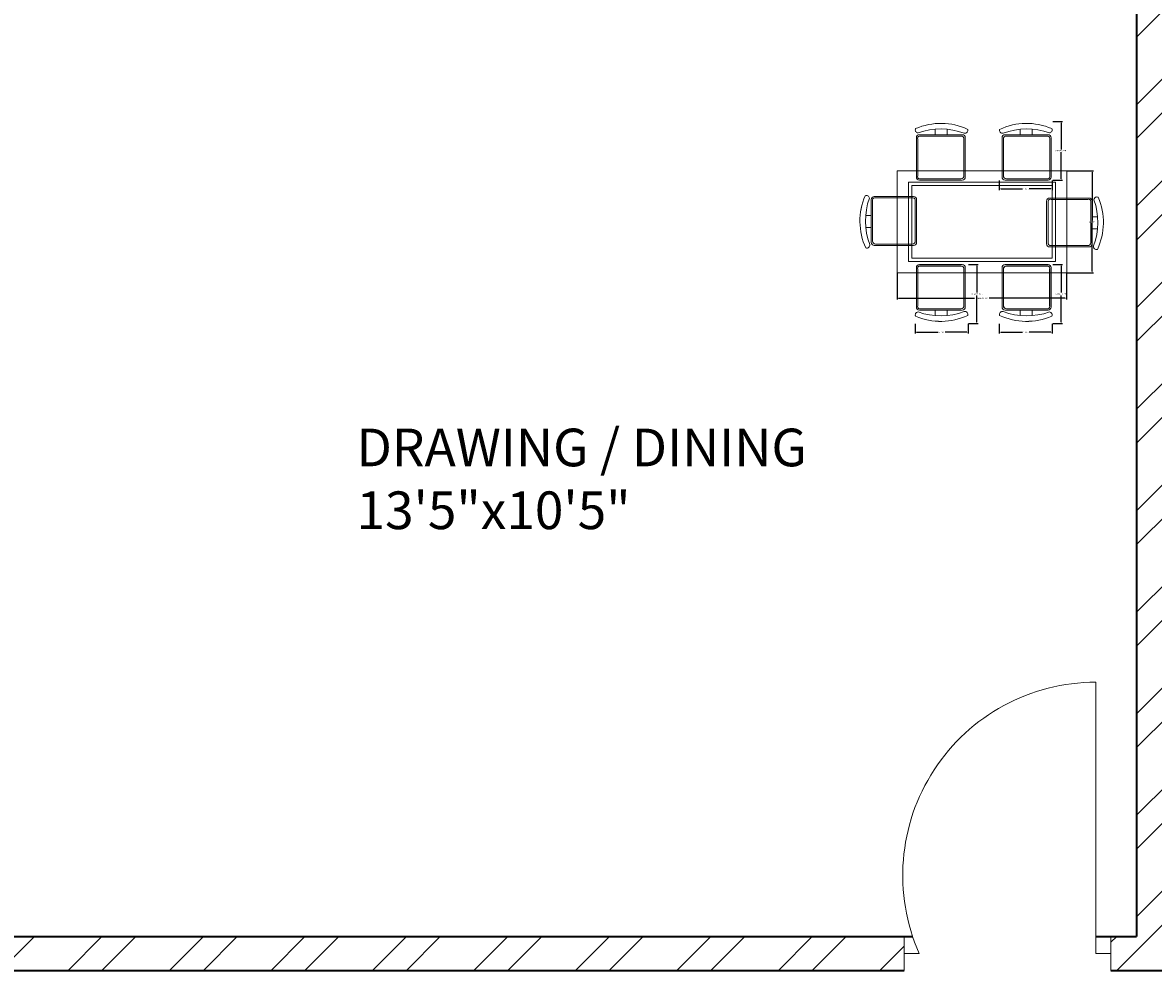
# Model space of a CAD drawing. Units: inches. Extents: x 1944 to 3454, y 1352 to 3055.
# Tile 6 of 17: x 2163 to 2314, y 1900 to 2026. Entities that reach past the tile are written whole.
import ezdxf

# ---------------------------------------------------------------- set-up
doc = ezdxf.new("R2010")
doc.units = ezdxf.units.IN
for name, color, linetype, lineweight in [('A-ANNO-DIMS', 2, 'Continuous', 18), ('A-AREA-IDEN', 7, 'Continuous', 18), ('A-DOOR', 3, 'Continuous', 20), ('A-FURN', 8, 'Continuous', 13), ('A-WALL', 7, 'Continuous', 35), ('A-WALL-PATT', 252, 'Continuous', 13)]:
    doc.layers.add(name, color=color, linetype=linetype, lineweight=lineweight)
doc.styles.get("Standard").update_dxf_attribs({"font": 'arial.ttf'})
doc.dimstyles.get("Standard").update_dxf_attribs({"dimtxt": 0.18, "dimasz": 0.18, "dimexe": 0.18, "dimexo": 0.0625, "dimgap": 0.09, "dimtad": 0, "dimtih": 1, "dimtoh": 1, "dimdec": 4, "dimzin": 0, "dimdsep": 46, "dimtxsty": 'Standard', "dimcen": 0.09, "dimadec": 0, "dimazin": 0, "dimtfac": 1, "dimtdec": 4, "dimtofl": 0, "dimtmove": 0, "dimatfit": 3, "dimfxl": 1, "dimtolj": 1, "dimtzin": 0, "dimarcsym": 0})

# ---------------------------------------------------------------- blocks, each defined once
blk = doc.blocks.new('DOOR-SWING-36IN-10')
for p, q in [((25.63, 2.25), (25.63, 38.25)), ((0.18, 4.5), (0.18, 0)), ((27.63, 4.5), (27.63, 0)), ((0.18, 0), (0.18, 2.25)), ((0.18, 2.25), (2.18, 2.25)), ((27.63, 2.25), (25.63, 2.25)), ((27.63, 0), (27.63, 2.25))]:
    blk.add_line(p, q)
blk.add_arc((25.63, 12.61), 25.64, 90, 203.8432)
blk = doc.blocks.new('TABLE-DINING-01')
for points in [[(0, 13.51), (22.52, 13.51), (22.52, 0), (0, 0)], [(0, 13.51), (22.52, 13.51), (22.52, 0), (0, 0)], [(1.5, 12.01), (21.02, 12.01), (21.02, 1.5), (1.5, 1.5)], [(1.5, 12.01), (21.02, 12.01), (21.02, 1.5), (1.5, 1.5)], [(1.95, 11.56), (20.57, 11.56), (20.57, 1.95), (1.95, 1.95)], [(1.95, 11.56), (20.57, 11.56), (20.57, 1.95), (1.95, 1.95)]]:
    blk.add_lwpolyline(points, close=True)
blk = doc.blocks.new('CHAIR-DINING-01')
for points in [[(0.48, 6.23, -0.578392), (0.02, 6.74, -0.214524), (6.94, 6.84, -0.552014), (6.62, 6.28, 0.175809), (0.48, 6.23)], [(6.44, 6.03, -0.414214), (6.84, 5.63), (6.84, 0.4, -0.414214), (6.44, 0), (0.74, 0, -0.414214), (0.34, 0.4), (0.34, 5.63, -0.414214), (0.74, 6.03), (6.44, 6.03)], [(2.74, 6.03), (2.74, 6.75, 0.064759)]]:
    blk.add_lwpolyline(points, format="xyb")
blk.add_lwpolyline([(4.34, 6.77), (4.34, 6.03)])
blk.add_lwpolyline([(6.44, 5.85), (0.92, 5.85, 0.414214), (0.52, 5.45), (0.52, 0.58, 0.414214), (0.92, 0.18), (6.44, 0.18, 0.512069), (6.66, 0.58), (6.66, 5.45, 0.512069)], format="xyb", close=True)
blk = doc.blocks.new('CHAIR-DINING-02')
for points in [[(0.48, 6.23, -0.578392), (0.02, 6.74, -0.214524), (6.94, 6.84, -0.552014), (6.62, 6.28, 0.175809), (0.48, 6.23)], [(6.44, 6.03, -0.414214), (6.84, 5.63), (6.84, 0.4, -0.414214), (6.44, 0), (0.74, 0, -0.414214), (0.34, 0.4), (0.34, 5.63, -0.414214), (0.74, 6.03), (6.44, 6.03)], [(2.74, 6.03), (2.74, 6.75, 0.064759)]]:
    blk.add_lwpolyline(points, format="xyb")
blk.add_lwpolyline([(4.34, 6.77), (4.34, 6.03)])
blk.add_lwpolyline([(6.44, 5.85), (0.92, 5.85, 0.414214), (0.52, 5.45), (0.52, 0.58, 0.414214), (0.92, 0.18), (6.44, 0.18, 0.512069), (6.66, 0.58), (6.66, 5.45, 0.512069)], format="xyb", close=True)
blk = doc.blocks.new('CHAIR-DINING-03')
for points in [[(6.03, 6.44, 0.414214), (5.63, 6.84), (0.4, 6.84, 0.414214), (0, 6.44), (0, 0.74, 0.414214), (0.4, 0.35), (5.63, 0.35, 0.414214), (6.03, 0.74), (6.03, 6.44)], [(6.28, 6.62, -0.175809), (6.23, 0.48, 0.578392), (6.74, 0.02, 0.214524), (6.84, 6.94, 0.552014), (6.28, 6.62, -0.065079)], [(6.03, 2.74), (6.75, 2.74, -0.064759)]]:
    blk.add_lwpolyline(points, format="xyb")
blk.add_lwpolyline([(5.85, 6.44), (5.85, 0.92, -0.414214), (5.45, 0.52), (0.58, 0.52, -0.414214), (0.18, 0.92), (0.18, 6.44, -0.512069), (0.58, 6.66), (5.45, 6.66, -0.512069)], format="xyb", close=True)
blk.add_lwpolyline([(6.77, 4.34), (6.03, 4.34)])
blk = doc.blocks.new('CHAIR-DINING-04')
for points in [[(6.24, 1.5), (0.55, 1.5, -0.414214), (0.15, 1.9), (0.15, 7.13, -0.414214), (0.55, 7.53), (6.24, 7.53, -0.414214), (6.64, 7.13), (6.64, 1.9, -0.414214), (6.24, 1.5)], [(6.5, 1.3, -0.578392), (6.97, 0.79, -0.214524), (0.04, 0.7, -0.552014), (0.37, 1.25, 0.175809), (6.5, 1.3)], [(4.24, 1.5), (4.24, 0.78, 0.064759)]]:
    blk.add_lwpolyline(points, format="xyb")
blk.add_lwpolyline([(0.55, 1.68), (6.06, 1.68, 0.414214), (6.46, 2.08), (6.46, 6.95, 0.414214), (6.06, 7.35), (0.55, 7.35, 0.512069), (0.33, 6.95), (0.33, 2.08, 0.512069)], format="xyb", close=True)
blk.add_lwpolyline([(2.65, 0.77), (2.65, 1.5)])
blk = doc.blocks.new('CHAIR-DINING-05')
for points in [[(6.44, 1.5, 0.414214), (6.84, 1.9), (6.84, 7.13, 0.414214), (6.44, 7.53), (0.74, 7.53, 0.414214), (0.34, 7.13), (0.34, 1.9, 0.414214), (0.74, 1.5), (6.44, 1.5)], [(6.62, 1.25, -0.175809), (0.48, 1.3, 0.578392), (0.02, 0.79, 0.214524), (6.94, 0.7, 0.552014), (6.62, 1.25, -0.065079)], [(2.74, 1.5), (2.74, 0.78, -0.064759)]]:
    blk.add_lwpolyline(points, format="xyb")
blk.add_lwpolyline([(6.44, 1.68), (0.92, 1.68, -0.414214), (0.52, 2.08), (0.52, 6.95, -0.414214), (0.92, 7.35), (6.44, 7.35, -0.512069), (6.66, 6.95), (6.66, 2.08, -0.512069)], format="xyb", close=True)
blk.add_lwpolyline([(4.34, 0.77), (4.34, 1.5)])
blk = doc.blocks.new('*D64')
at = {"layer": 'A-ANNO-DIMS', "color": 0, "lineweight": -2, "transparency": 16777216}
for p, q in [((2279.54, 1992.61), (2279.54, 1989.12)), ((2302.06, 1992.61), (2302.06, 1989.12)), ((2279.72, 1989.3), (2289.84, 1989.3)), ((2301.88, 1989.3), (2291.77, 1989.3))]:
    blk.add_line(p, q, dxfattribs=at)
at = {"layer": 'A-ANNO-DIMS', "color": 0, "transparency": 16777216}
for points in [[(2279.72, 1989.33), (2279.72, 1989.27), (2279.54, 1989.3)], [(2301.88, 1989.33), (2301.88, 1989.27), (2302.06, 1989.3)]]:
    blk.add_solid(points, dxfattribs=at)
at = {"layer": 'Defpoints', "color": 0, "transparency": 16777216}
for p in [(2279.54, 1992.68), (2302.06, 1992.68), (2302.06, 1989.3)]:
    blk.add_point(p, dxfattribs=at)
at = {"layer": 'A-ANNO-DIMS', "color": 0, "transparency": 16777216, "insert": (2290.8, 1989.3), "char_height": 0.18, "attachment_point": 5}
blk.add_mtext('\\A1;TABLE 23 TYP.', dxfattribs=at)
blk = doc.blocks.new('*D65')
at = {"layer": 'A-ANNO-DIMS', "color": 0, "lineweight": -2, "transparency": 16777216}
for p, q in [((2302.13, 2006.19), (2305.62, 2006.19)), ((2305.44, 2006.01), (2305.44, 1999.61)), ((2305.44, 1992.86), (2305.44, 1999.25)), ((2302.13, 1992.68), (2305.62, 1992.68))]:
    blk.add_line(p, q, dxfattribs=at)
at = {"layer": 'A-ANNO-DIMS', "color": 0, "transparency": 16777216}
for points in [[(2305.41, 2006.01), (2305.47, 2006.01), (2305.44, 2006.19)], [(2305.41, 1992.86), (2305.47, 1992.86), (2305.44, 1992.68)]]:
    blk.add_solid(points, dxfattribs=at)
at = {"layer": 'Defpoints', "color": 0, "transparency": 16777216}
for p in [(2302.06, 2006.19), (2305.44, 2006.19), (2302.06, 1992.68)]:
    blk.add_point(p, dxfattribs=at)
at = {"layer": 'A-ANNO-DIMS', "color": 0, "transparency": 16777216, "insert": (2305.44, 1999.43), "char_height": 0.18, "attachment_point": 5}
blk.add_mtext('\\A1;14 TYP.', dxfattribs=at)
blk = doc.blocks.new('*D140')
at = {"layer": 'A-ANNO-DIMS', "color": 0, "lineweight": -2, "transparency": 16777216}
for p, q in [((2300.21, 2012.76), (2301.5, 2012.76)), ((2301.32, 2012.58), (2301.32, 2009.05)), ((2301.32, 2005.14), (2301.32, 2008.68)), ((2300.21, 2004.96), (2301.5, 2004.96))]:
    blk.add_line(p, q, dxfattribs=at)
at = {"layer": 'A-ANNO-DIMS', "color": 0, "transparency": 16777216}
for points in [[(2301.29, 2012.58), (2301.35, 2012.58), (2301.32, 2012.76)], [(2301.29, 2005.14), (2301.35, 2005.14), (2301.32, 2004.96)]]:
    blk.add_solid(points, dxfattribs=at)
at = {"layer": 'Defpoints', "color": 0, "transparency": 16777216}
for p in [(2300.15, 2012.76), (2301.32, 2012.76), (2300.15, 2004.96)]:
    blk.add_point(p, dxfattribs=at)
at = {"layer": 'A-ANNO-DIMS', "color": 0, "transparency": 16777216, "insert": (2301.32, 2008.86), "char_height": 0.18, "attachment_point": 5}
blk.add_mtext('\\A1;CHAIR 8 TYP.', dxfattribs=at)
blk = doc.blocks.new('*D141')
at = {"layer": 'A-ANNO-DIMS', "color": 0, "lineweight": -2, "transparency": 16777216}
for p, q in [((2293.12, 2004.9), (2293.12, 2003.62)), ((2300.15, 2004.9), (2300.15, 2003.62)), ((2293.3, 2003.8), (2296.18, 2003.8)), ((2299.97, 2003.8), (2297.09, 2003.8))]:
    blk.add_line(p, q, dxfattribs=at)
at = {"layer": 'A-ANNO-DIMS', "color": 0, "transparency": 16777216}
for points in [[(2293.3, 2003.83), (2293.3, 2003.77), (2293.12, 2003.8)], [(2299.97, 2003.83), (2299.97, 2003.77), (2300.15, 2003.8)]]:
    blk.add_solid(points, dxfattribs=at)
at = {"layer": 'Defpoints', "color": 0, "transparency": 16777216}
for p in [(2293.12, 2004.96), (2300.15, 2004.96), (2300.15, 2003.8)]:
    blk.add_point(p, dxfattribs=at)
at = {"layer": 'A-ANNO-DIMS', "color": 0, "transparency": 16777216, "insert": (2296.63, 2003.8), "char_height": 0.18, "attachment_point": 5}
blk.add_mtext('\\A1;7 TYP.', dxfattribs=at)
blk = doc.blocks.new('*D146')
at = {"layer": 'A-ANNO-DIMS', "color": 0, "lineweight": -2, "transparency": 16777216}
for p, q in [((2289.03, 1993.76), (2290.32, 1993.76)), ((2290.14, 1993.58), (2290.14, 1990.04)), ((2290.14, 1986.14), (2290.14, 1989.67)), ((2289.03, 1985.96), (2290.32, 1985.96))]:
    blk.add_line(p, q, dxfattribs=at)
at = {"layer": 'A-ANNO-DIMS', "color": 0, "transparency": 16777216}
for points in [[(2290.11, 1993.58), (2290.17, 1993.58), (2290.14, 1993.76)], [(2290.11, 1986.14), (2290.17, 1986.14), (2290.14, 1985.96)]]:
    blk.add_solid(points, dxfattribs=at)
at = {"layer": 'Defpoints', "color": 0, "transparency": 16777216}
for p in [(2288.97, 1993.76), (2290.14, 1993.76), (2288.97, 1985.96)]:
    blk.add_point(p, dxfattribs=at)
at = {"layer": 'A-ANNO-DIMS', "color": 0, "transparency": 16777216, "insert": (2290.14, 1989.86), "char_height": 0.18, "attachment_point": 5}
blk.add_mtext('\\A1;CHAIR 8 TYP.', dxfattribs=at)
blk = doc.blocks.new('*D147')
at = {"layer": 'A-ANNO-DIMS', "color": 0, "lineweight": -2, "transparency": 16777216}
for p, q in [((2281.94, 1985.9), (2281.94, 1984.61)), ((2288.97, 1985.9), (2288.97, 1984.61)), ((2282.12, 1984.79), (2285, 1984.79)), ((2288.79, 1984.79), (2285.92, 1984.79))]:
    blk.add_line(p, q, dxfattribs=at)
at = {"layer": 'A-ANNO-DIMS', "color": 0, "transparency": 16777216}
for points in [[(2282.12, 1984.82), (2282.12, 1984.76), (2281.94, 1984.79)], [(2288.79, 1984.82), (2288.79, 1984.76), (2288.97, 1984.79)]]:
    blk.add_solid(points, dxfattribs=at)
at = {"layer": 'Defpoints', "color": 0, "transparency": 16777216}
for p in [(2281.94, 1985.96), (2288.97, 1985.96), (2288.97, 1984.79)]:
    blk.add_point(p, dxfattribs=at)
at = {"layer": 'A-ANNO-DIMS', "color": 0, "transparency": 16777216, "insert": (2285.46, 1984.79), "char_height": 0.18, "attachment_point": 5}
blk.add_mtext('\\A1;7 TYP.', dxfattribs=at)
blk = doc.blocks.new('*D148')
at = {"layer": 'A-ANNO-DIMS', "color": 0, "lineweight": -2, "transparency": 16777216}
for p, q in [((2300.21, 1993.76), (2301.5, 1993.76)), ((2301.32, 1993.58), (2301.32, 1990.04)), ((2301.32, 1986.14), (2301.32, 1989.67)), ((2300.21, 1985.96), (2301.5, 1985.96))]:
    blk.add_line(p, q, dxfattribs=at)
at = {"layer": 'A-ANNO-DIMS', "color": 0, "transparency": 16777216}
for points in [[(2301.29, 1993.58), (2301.35, 1993.58), (2301.32, 1993.76)], [(2301.29, 1986.14), (2301.35, 1986.14), (2301.32, 1985.96)]]:
    blk.add_solid(points, dxfattribs=at)
at = {"layer": 'Defpoints', "color": 0, "transparency": 16777216}
for p in [(2300.15, 1993.76), (2301.32, 1993.76), (2300.15, 1985.96)]:
    blk.add_point(p, dxfattribs=at)
at = {"layer": 'A-ANNO-DIMS', "color": 0, "transparency": 16777216, "insert": (2301.32, 1989.86), "char_height": 0.18, "attachment_point": 5}
blk.add_mtext('\\A1;CHAIR 8 TYP.', dxfattribs=at)
blk = doc.blocks.new('*D149')
at = {"layer": 'A-ANNO-DIMS', "color": 0, "lineweight": -2, "transparency": 16777216}
for p, q in [((2293.12, 1985.9), (2293.12, 1984.61)), ((2300.15, 1985.9), (2300.15, 1984.61)), ((2293.3, 1984.79), (2296.18, 1984.79)), ((2299.97, 1984.79), (2297.09, 1984.79))]:
    blk.add_line(p, q, dxfattribs=at)
at = {"layer": 'A-ANNO-DIMS', "color": 0, "transparency": 16777216}
for points in [[(2293.3, 1984.82), (2293.3, 1984.76), (2293.12, 1984.79)], [(2299.97, 1984.82), (2299.97, 1984.76), (2300.15, 1984.79)]]:
    blk.add_solid(points, dxfattribs=at)
at = {"layer": 'Defpoints', "color": 0, "transparency": 16777216}
for p in [(2293.12, 1985.96), (2300.15, 1985.96), (2300.15, 1984.79)]:
    blk.add_point(p, dxfattribs=at)
at = {"layer": 'A-ANNO-DIMS', "color": 0, "transparency": 16777216, "insert": (2296.63, 1984.79), "char_height": 0.18, "attachment_point": 5}
blk.add_mtext('\\A1;7 TYP.', dxfattribs=at)

msp = doc.modelspace()

# ---------------------------------------------------------------- hatches: boundary and pattern name
at = {"layer": 'A-WALL-PATT'}
h = msp.add_hatch(dxfattribs=at)
h.set_pattern_fill('ANSI32', color=256)
h.paths.add_polyline_path([(2061.822, 2177.596), (2158.181, 2177.596), (2158.181, 2179.846), (2158.181, 2182.096), (2057.322, 2182.096), (2057.322, 2123.452), (2061.822, 2123.452)])
h.paths.add_polyline_path([(2258.993, 2179.846), (2258.993, 2182.096), (2218.838, 2182.096), (2218.838, 2177.596), (2258.993, 2177.596)])
h.paths.add_polyline_path([(2315.822, 2177.596), (2322.722, 2177.596), (2322.722, 2182.096), (2303.186, 2182.096), (2303.186, 2177.596), (2311.322, 2177.596), (2311.322, 2033.596), (2231.355, 2033.596), (2231.355, 2029.096), (2311.322, 2029.096), (2311.322, 1904.596), (2307.941, 1904.596), (2307.941, 1900.096), (2319.277, 1900.096), (2319.277, 1902.346), (2319.277, 1904.596), (2315.822, 1904.596), (2315.822, 2029.096), (2394.855, 2029.096), (2394.855, 2033.596), (2315.822, 2033.596)])
h.paths.add_polyline_path([(2407.334, 2182.096), (2366.1, 2182.096), (2366.1, 2177.596), (2407.334, 2177.596), (2407.334, 2179.846)])
h.paths.add_polyline_path([(2440.322, 2177.596), (2443.866, 2177.596), (2443.866, 2182.096), (2431.827, 2182.096), (2431.827, 2179.846), (2431.827, 2177.596), (2435.822, 2177.596), (2435.822, 2033.596), (2430.464, 2033.596), (2430.464, 2029.096), (2445.372, 2029.096), (2445.372, 2031.346), (2445.372, 2033.596), (2440.322, 2033.596)])
h.paths.add_polyline_path([(2569.822, 2182.096), (2466.481, 2182.096), (2466.481, 2177.596), (2565.322, 2177.596), (2565.322, 2123.452), (2569.822, 2123.452)])
h.paths.add_polyline_path([(2569.822, 2063.452), (2567.572, 2063.452), (2565.322, 2063.452), (2565.322, 2033.596), (2478.08, 2033.596), (2476.822, 2033.596), (2476.822, 2028.698), (2476.822, 2020.069), (2481.322, 2020.069), (2481.322, 2029.096), (2565.322, 2029.096), (2565.322, 2014.5), (2569.822, 2014.5)])
h.paths.add_polyline_path([(2569.822, 1978.5), (2565.322, 1978.5), (2565.322, 1957.096), (2481.322, 1957.096), (2481.322, 1990.369), (2476.822, 1990.369), (2476.822, 1957.096), (2476.822, 1952.596), (2476.822, 1947.471), (2481.322, 1947.471), (2481.322, 1952.596), (2565.322, 1952.596), (2565.322, 1943.2), (2569.822, 1943.2)])
h.paths.add_polyline_path([(2569.822, 1919.2), (2565.322, 1919.2), (2565.322, 1904.596), (2481.322, 1904.596), (2481.322, 1928.596), (2476.822, 1928.596), (2476.822, 1904.596), (2350.518, 1904.596), (2350.518, 1900.096), (2476.822, 1900.096), (2565.322, 1900.096), (2565.322, 1895.596), (2565.322, 1887.047), (2569.822, 1887.047)])
h.paths.add_polyline_path([(2280.492, 1904.596), (2150.322, 1904.596), (2150.322, 1926.68), (2148.072, 1926.68), (2145.822, 1926.68), (2145.822, 1904.596), (2061.822, 1904.596), (2061.822, 1914.977), (2059.572, 1914.977), (2057.322, 1914.977), (2057.322, 1887.362), (2061.822, 1887.362), (2061.822, 1900.096), (2150.322, 1900.096), (2280.492, 1900.096), (2280.492, 1902.346)])
h.paths.add_polyline_path([(2150.322, 1957.096), (2150.322, 1986.22), (2145.822, 1986.22), (2145.822, 1957.096), (2061.822, 1957.096), (2061.822, 1975.678), (2057.322, 1975.678), (2057.322, 1938.977), (2061.822, 1938.977), (2061.822, 1952.596), (2145.822, 1952.596), (2145.822, 1947.985), (2150.322, 1947.985), (2150.322, 1952.596)])
h.paths.add_polyline_path([(2061.822, 2063.452), (2057.322, 2063.452), (2057.322, 2011.678), (2061.822, 2011.678), (2061.822, 2029.096), (2145.288, 2029.096), (2145.822, 2029.096), (2145.822, 2019.118), (2150.322, 2019.118), (2150.322, 2029.096), (2150.322, 2033.596), (2147.022, 2033.596), (2061.822, 2033.596)])
h.paths.add_polyline_path([(2061.822, 1835.596), (2133.822, 1835.596), (2133.822, 1794.415), (2138.322, 1794.415), (2138.322, 1835.596), (2231.726, 1835.596), (2231.726, 1840.096), (2061.822, 1840.096), (2061.822, 1851.362), (2057.322, 1851.362), (2057.322, 1810.528), (2061.822, 1810.528)])
h.paths.add_polyline_path([(2061.822, 1774.528), (2059.572, 1774.528), (2057.322, 1774.528), (2057.322, 1723.746), (2061.822, 1723.746), (2061.822, 1735.096), (2133.822, 1735.096), (2133.822, 1731.415), (2138.322, 1731.415), (2138.322, 1759.737), (2133.822, 1759.737), (2133.822, 1739.596), (2061.822, 1739.596)])
h.paths.add_polyline_path([(2061.822, 1678.596), (2147.597, 1678.596), (2147.597, 1680.846), (2147.597, 1683.096), (2138.322, 1683.096), (2138.322, 1710.66), (2136.072, 1710.66), (2133.822, 1710.66), (2133.822, 1683.096), (2061.822, 1683.096), (2061.822, 1699.746), (2057.322, 1699.746), (2057.322, 1645.751), (2061.822, 1645.751)])
h.paths.add_polyline_path([(2061.822, 1585.751), (2057.322, 1585.751), (2057.322, 1530.096), (2158.703, 1530.096), (2158.703, 1534.596), (2061.822, 1534.596)])
h.paths.add_polyline_path([(2191.322, 1678.596), (2195.889, 1678.596), (2195.889, 1683.096), (2181.763, 1683.096), (2181.763, 1680.846), (2181.763, 1678.596), (2186.822, 1678.596), (2186.822, 1534.596), (2181.354, 1534.596), (2181.354, 1530.096), (2196.54, 1530.096), (2196.54, 1532.346), (2196.54, 1534.596), (2191.322, 1534.596)])
h.paths.add_polyline_path([(2315.822, 1678.596), (2402.014, 1678.596), (2402.014, 1683.096), (2355.822, 1683.096), (2355.822, 1835.596), (2360.838, 1835.596), (2360.838, 1840.096), (2351.322, 1840.096), (2351.322, 1683.096), (2273.322, 1683.096), (2273.322, 1840.096), (2263.134, 1840.096), (2263.134, 1837.846), (2263.134, 1835.596), (2268.822, 1835.596), (2268.822, 1683.096), (2227.793, 1683.096), (2227.793, 1678.596), (2311.322, 1678.596), (2311.322, 1534.596), (2302.384, 1534.596), (2302.384, 1530.096), (2324.521, 1530.096), (2324.521, 1532.346), (2324.521, 1534.596), (2315.822, 1534.596)])
h.paths.add_polyline_path([(2440.322, 1678.596), (2443.656, 1678.596), (2443.656, 1683.096), (2432.614, 1683.096), (2432.614, 1680.846), (2432.614, 1678.596), (2435.822, 1678.596), (2435.822, 1534.596), (2440.322, 1534.596)])
h.paths.add_polyline_path([(2409.913, 1534.596), (2369.033, 1534.596), (2369.033, 1530.096), (2409.913, 1530.096)])
h.paths.add_polyline_path([(2259.529, 1532.346), (2259.529, 1534.596), (2218.889, 1534.596), (2218.889, 1532.346), (2218.889, 1530.096), (2259.529, 1530.096)])
h.paths.add_polyline_path([(2569.822, 1584.389), (2567.572, 1584.389), (2565.322, 1584.389), (2565.322, 1534.596), (2465.892, 1534.596), (2465.892, 1530.096), (2569.822, 1530.096)])
h.paths.add_polyline_path([(2505.567, 1530.096), (2501.067, 1530.096), (2501.067, 1494.096), (2381.067, 1494.096), (2381.067, 1530.096), (2376.567, 1530.096), (2376.567, 1489.596), (2381.067, 1489.596), (2505.567, 1489.596), (2505.567, 1494.096)])
h.paths.add_polyline_path([(2127.673, 1530.096), (2123.173, 1530.096), (2123.173, 1489.596), (2127.673, 1489.596), (2252.173, 1489.596), (2252.173, 1494.096), (2252.173, 1530.096), (2247.673, 1530.096), (2247.673, 1494.096), (2127.673, 1494.096)])
h.paths.add_polyline_path([(2251.167, 2222.596), (2126.667, 2222.596), (2122.167, 2222.596), (2122.167, 2182.096), (2126.667, 2182.096), (2126.667, 2218.096), (2210.667, 2218.096), (2234.667, 2218.096), (2246.667, 2218.096), (2246.667, 2182.096), (2251.167, 2182.096), (2251.167, 2218.096)])
h.paths.add_polyline_path([(2501.916, 2222.596), (2497.416, 2222.596), (2372.916, 2222.596), (2372.916, 2218.096), (2372.916, 2182.096), (2377.416, 2182.096), (2377.416, 2218.096), (2497.416, 2218.096), (2497.416, 2182.096), (2501.916, 2182.096)])
h.paths.add_polyline_path([(2569.822, 1700.442), (2565.322, 1700.442), (2565.322, 1683.096), (2493.322, 1683.096), (2493.322, 1709.096), (2488.822, 1709.096), (2488.822, 1683.096), (2475.416, 1683.096), (2475.416, 1680.846), (2475.416, 1678.596), (2488.822, 1678.596), (2565.322, 1678.596), (2565.322, 1644.389), (2569.822, 1644.389)])
h.paths.add_polyline_path([(2569.822, 1773.506), (2565.322, 1773.506), (2565.322, 1739.596), (2493.322, 1739.596), (2493.322, 1754.002), (2488.822, 1754.002), (2488.822, 1729.846), (2491.072, 1729.846), (2493.322, 1729.846), (2493.322, 1735.096), (2565.322, 1735.096), (2565.322, 1724.442), (2569.822, 1724.442)])
h.paths.add_polyline_path([(2569.822, 1851.047), (2567.572, 1851.047), (2565.322, 1851.047), (2565.322, 1840.096), (2395.039, 1840.096), (2395.039, 1837.846), (2395.039, 1835.596), (2488.822, 1835.596), (2488.822, 1798.423), (2493.322, 1798.423), (2493.322, 1835.596), (2565.322, 1835.596), (2565.322, 1809.506), (2569.822, 1809.506)])
h.paths.add_polyline_path([(2347.275, 1955.576), (2414.024, 1955.576), (2414.024, 1974.234), (2347.275, 1974.234)], flags=9)
h.paths.add_polyline_path([(2509.756, 1990.497), (2542.915, 1990.497), (2542.915, 2009.154), (2509.756, 2009.154)], flags=9)

# ---------------------------------------------------------------- linework, layer by layer
at = {"layer": 'A-FURN'}
for points in [[(2282.33, 2011.244, -0.1758092), (2288.464, 2011.197, 0.5783921), (2288.929, 2011.708, 0.2145244), (2282.005, 2011.801, 0.552014), (2282.33, 2011.244, -0.065079)], [(2282.33, 2011.244, -0.1758092), (2288.464, 2011.197, 0.5783921), (2288.929, 2011.708, 0.2145244), (2282.005, 2011.801, 0.552014), (2282.33, 2011.244, -0.065079)], [(2286.204, 2010.998), (2286.204, 2011.718, -0.0647586)], [(2286.204, 2010.997), (2286.204, 2011.718, -0.0647586)], [(2288.204, 2010.998), (2282.509, 2010.998, 0.4142136), (2282.111, 2010.599), (2282.111, 2005.363, 0.4142136), (2282.509, 2004.965), (2288.204, 2004.965, 0.4142136), (2288.602, 2005.363), (2288.602, 2010.599, 0.4142136), (2288.204, 2010.998)], [(2288.204, 2010.997), (2282.509, 2010.997, 0.4142136), (2282.111, 2010.599), (2282.111, 2005.363, 0.4142136), (2282.509, 2004.965), (2288.204, 2004.965, 0.4142136), (2288.602, 2005.363), (2288.602, 2010.599, 0.4142136), (2288.204, 2010.997)], [(2275.913, 1996.431, -0.5783921), (2275.402, 1995.967, -0.2145244), (2275.309, 2002.891, -0.552014), (2275.867, 2002.565, 0.1758094), (2275.913, 1996.431)], [(2275.913, 1996.431, -0.5783921), (2275.402, 1995.967, -0.2145244), (2275.309, 2002.89, -0.552014), (2275.867, 2002.565, 0.1758094), (2275.913, 1996.431)], [(2276.113, 2002.386, -0.4142136), (2276.511, 2002.785), (2281.747, 2002.785, -0.4142136), (2282.146, 2002.386), (2282.146, 1996.692, -0.4142136), (2281.747, 1996.293), (2276.511, 1996.293, -0.4142136), (2276.113, 1996.692), (2276.113, 2002.386)], [(2276.113, 2002.386, -0.4142136), (2276.511, 2002.784), (2281.747, 2002.784, -0.4142136), (2282.146, 2002.386), (2282.146, 1996.691, -0.4142136), (2281.747, 1996.293), (2276.511, 1996.293, -0.4142136), (2276.113, 1996.691), (2276.113, 2002.386)], [(2305.437, 2002.191, 0.4142136), (2305.038, 2002.589), (2299.802, 2002.589, 0.4142136), (2299.404, 2002.191), (2299.404, 1996.496, 0.4142136), (2299.802, 1996.098), (2305.038, 1996.098, 0.4142136), (2305.437, 1996.496), (2305.437, 2002.191)], [(2305.683, 2002.37, -0.1758092), (2305.636, 1996.236, 0.5783921), (2306.147, 1995.772, 0.2145244), (2306.24, 2002.695, 0.552014), (2305.683, 2002.37, -0.065079)], [(2276.113, 1998.692), (2275.393, 1998.692, 0.0647586)], [(2276.113, 1998.692), (2275.393, 1998.692, 0.0647586)], [(2305.437, 1998.497), (2306.157, 1998.497, -0.0647586)], [(2288.204, 1987.722), (2282.509, 1987.722, -0.4142136), (2282.111, 1988.121), (2282.111, 1993.357, -0.4142136), (2282.509, 1993.755), (2288.204, 1993.755, -0.4142136), (2288.602, 1993.357), (2288.602, 1988.121, -0.4142136), (2288.204, 1987.722)], [(2299.583, 1987.722, 0.4142136), (2299.981, 1988.121), (2299.981, 1993.357, 0.4142136), (2299.583, 1993.755), (2293.888, 1993.755, 0.4142136), (2293.49, 1993.357), (2293.49, 1988.121, 0.4142136), (2293.888, 1987.722), (2299.583, 1987.722)], [(2288.464, 1987.523, -0.5783921), (2288.929, 1987.012, -0.2145244), (2282.005, 1986.919, -0.552014), (2282.33, 1987.476, 0.1758093), (2288.464, 1987.523)], [(2286.204, 1987.722), (2286.204, 1987.002, 0.0647586)], [(2299.762, 1987.476, -0.1758093), (2293.628, 1987.523, 0.5783921), (2293.163, 1987.012, 0.2145244), (2300.087, 1986.919, 0.552014), (2299.762, 1987.476, -0.065079)], [(2295.889, 1987.722), (2295.889, 1987.002, -0.0647586)]]:
    msp.add_lwpolyline(points, format="xyb", dxfattribs=at)
for points in [[(2284.61, 2011.731), (2284.61, 2010.998)], [(2284.61, 2011.731), (2284.61, 2010.997)], [(2275.38, 2000.286), (2276.113, 2000.286)], [(2275.38, 2000.286), (2276.113, 2000.286)], [(2306.17, 2000.091), (2305.437, 2000.091)], [(2284.61, 1986.989), (2284.61, 1987.722)], [(2297.482, 1986.989), (2297.482, 1987.722)]]:
    msp.add_lwpolyline(points, dxfattribs=at)
for points in [[(2282.512, 2010.818), (2288.024, 2010.818, -0.4142136), (2288.423, 2010.42), (2288.423, 2005.543, -0.4142136), (2288.024, 2005.144), (2282.512, 2005.144, -0.5120695), (2282.291, 2005.543), (2282.291, 2010.42, -0.5120695)], [(2282.512, 2010.818), (2288.024, 2010.818, -0.4142136), (2288.423, 2010.42), (2288.423, 2005.543, -0.4142136), (2288.024, 2005.144), (2282.512, 2005.144, -0.5120695), (2282.291, 2005.543), (2282.291, 2010.42, -0.5120695)], [(2276.292, 2002.384), (2276.292, 1996.871, 0.4142136), (2276.691, 1996.473), (2281.568, 1996.473, 0.4142136), (2281.966, 1996.871), (2281.966, 2002.384, 0.5120695), (2281.568, 2002.605), (2276.691, 2002.605, 0.5120695)], [(2276.292, 2002.384), (2276.292, 1996.871, 0.4142136), (2276.691, 1996.473), (2281.568, 1996.473, 0.4142136), (2281.966, 1996.871), (2281.966, 2002.384, 0.5120695), (2281.568, 2002.605), (2276.691, 2002.605, 0.5120695)], [(2305.257, 2002.189), (2305.257, 1996.676, -0.4142136), (2304.859, 1996.278), (2299.982, 1996.278, -0.4142136), (2299.583, 1996.676), (2299.583, 2002.189, -0.5120695), (2299.982, 2002.41), (2304.859, 2002.41, -0.5120695)], [(2282.512, 1987.902), (2288.024, 1987.902, 0.4142136), (2288.423, 1988.3), (2288.423, 1993.177, 0.4142136), (2288.024, 1993.576), (2282.512, 1993.576, 0.5120695), (2282.291, 1993.177), (2282.291, 1988.3, 0.5120695)], [(2299.58, 1987.902), (2294.068, 1987.902, -0.4142136), (2293.669, 1988.3), (2293.669, 1993.177, -0.4142136), (2294.068, 1993.576), (2299.58, 1993.576, -0.5120695), (2299.802, 1993.177), (2299.802, 1988.3, -0.5120695)]]:
    msp.add_lwpolyline(points, format="xyb", close=True, dxfattribs=at)
at = {"layer": 'A-WALL'}
for p, q in [((2311.322, 2029.096), (2311.322, 1904.596)), ((2150.322, 1904.596), (2281.622, 1904.596)), ((2305.941, 1904.596), (2311.322, 1904.596)), ((2150.322, 1900.096), (2280.492, 1900.096)), ((2307.941, 1900.096), (2319.277, 1900.096))]:
    msp.add_line(p, q, dxfattribs=at)

# ---------------------------------------------------------------- block references
at = {"layer": 'A-DOOR'}
msp.add_blockref('DOOR-SWING-36IN-10', (2280.309, 1900.096), dxfattribs=at)
at = {"layer": 'A-FURN'}
for name, p in [('CHAIR-DINING-01', (2293.145, 2004.965)), ('CHAIR-DINING-02', (2293.145, 2004.965)), ('TABLE-DINING-01', (2279.545, 1992.676)), ('CHAIR-DINING-03', (2299.404, 1995.753)), ('CHAIR-DINING-04', (2281.962, 1986.223)), ('CHAIR-DINING-05', (2293.145, 1986.223))]:
    msp.add_blockref(name, p, dxfattribs=at)

# ---------------------------------------------------------------- texts
at = {"layer": 'A-AREA-IDEN', "insert": (2207.796, 1971.99), "char_height": 5, "attachment_point": 1}
msp.add_mtext_dynamic_manual_height_columns('DRAWING / DINING\\P13\'5"x10\'5"', width=182.48881, gutter_width=12.5, heights=[0], dxfattribs=at)

# ---------------------------------------------------------------- dimensions: what is measured, and where the dimension line sits
at = {"layer": 'A-ANNO-DIMS'}
for base, p1, p2, text, picture, middle in [((2301.317, 2012.762), (2300.148, 2004.965), (2300.148, 2012.762), 'CHAIR <> TYP.', '*D140', (2301.317, 2008.863)), ((2305.443, 2006.189), (2302.065, 1992.676), (2302.065, 2006.189), '<> TYP.', '*D65', (2305.443, 1999.432)), ((2290.142, 1993.755), (2288.972, 1985.958), (2288.972, 1993.755), 'CHAIR <> TYP.', '*D146', (2290.142, 1989.857)), ((2301.317, 1993.755), (2300.148, 1985.958), (2300.148, 1993.755), 'CHAIR <> TYP.', '*D148', (2301.317, 1989.857))]:
    dim = msp.add_linear_dim(base=base, p1=p1, p2=p2, angle=90, text=text, dimstyle='Standard', override={"dimdec": 0, "dimlfac": 1, "dimrnd": 0, "dimzin": 0, "dimdsep": 46, "dimlunit": 2}, dxfattribs=at)
    dim.commit()
    dim.dimension.update_dxf_attribs({"geometry": picture, "text_midpoint": middle})
for base, p1, p2, text, picture, middle in [((2300.148, 2003.795), (2293.12, 2004.965), (2300.148, 2004.965), '<> TYP.', '*D141', (2296.634, 2003.795)), ((2302.065, 1989.298), (2279.545, 1992.676), (2302.065, 1992.676), 'TABLE <> TYP.', '*D64', (2290.805, 1989.298)), ((2288.972, 1984.789), (2281.944, 1985.958), (2288.972, 1985.958), '<> TYP.', '*D147', (2285.458, 1984.789)), ((2300.148, 1984.789), (2293.12, 1985.958), (2300.148, 1985.958), '<> TYP.', '*D149', (2296.634, 1984.789))]:
    dim = msp.add_linear_dim(base=base, p1=p1, p2=p2, text=text, dimstyle='Standard', override={"dimdec": 0, "dimlfac": 1, "dimrnd": 0, "dimzin": 0, "dimdsep": 46, "dimlunit": 2}, dxfattribs=at)
    dim.commit()
    dim.dimension.update_dxf_attribs({"geometry": picture, "text_midpoint": middle})

doc.saveas('drawing.dxf')
